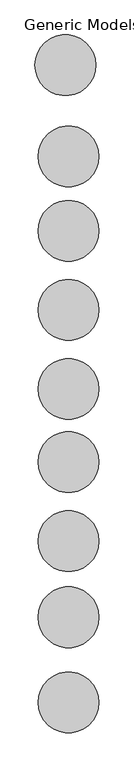
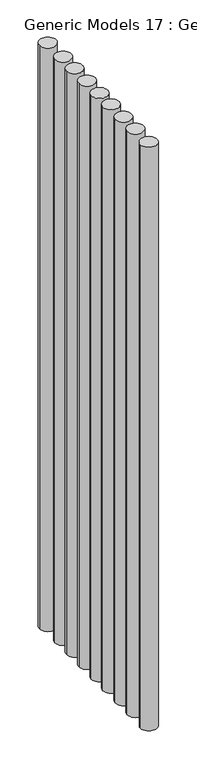
"""IFC4 building model written with IfcOpenShell, lengths in millimetres: proxy geometry, Generic Models 17 : Generic Models 17."""

from ifc_helpers import new_model, si_unit, point, frame, frame_2d, origin, place, context, project, spatial, circle_curve, trimmed, segment, composite_curve, outline, extrude, source, transform, mapped, element, save


def generic_models_17_generic_models_17_6d1cac68(model_context):
    return source(origin(), model_context, "Body", "SweptSolid", [
        extrude(outline(composite_curve([segment(trimmed(circle_curve(frame_2d((-2170.5790175, 11540.1337355)), 63.5), [point((-2234.0790175, 11540.1337355))], [point((-2107.0790175, 11540.1337355))], False, "CARTESIAN"), True, "CONTINUOUS"), segment(trimmed(circle_curve(frame_2d((-2170.5790175, 11540.1337355)), 63.5), [point((-2107.0790175, 11540.1337355))], [point((-2234.0790175, 11540.1337355))], False, "CARTESIAN"), True, "CONTINUOUS")], self_intersect=False)), frame((0.0, 0.0, 457.2), z_axis=(0.0, 0.0, 1.0), x_axis=(1.0, 0.0, 0.0)), (0.0, 0.0, 1.0), 4724.4),
        extrude(outline(composite_curve([segment(trimmed(circle_curve(frame_2d((-2163.9306633, 11349.749783)), 63.5), [point((-2227.4306633, 11349.749783))], [point((-2100.4306633, 11349.749783))], False, "CARTESIAN"), True, "CONTINUOUS"), segment(trimmed(circle_curve(frame_2d((-2163.9306633, 11349.749783)), 63.5), [point((-2100.4306633, 11349.749783))], [point((-2227.4306633, 11349.749783))], False, "CARTESIAN"), True, "CONTINUOUS")], self_intersect=False)), frame((0.0, 0.0, 457.2), z_axis=(0.0, 0.0, 1.0), x_axis=(1.0, 0.0, 0.0)), (0.0, 0.0, 1.0), 4724.4),
        extrude(outline(composite_curve([segment(trimmed(circle_curve(frame_2d((-2163.9306633, 11194.406573)), 63.5), [point((-2227.4306633, 11194.406573))], [point((-2100.4306633, 11194.406573))], False, "CARTESIAN"), True, "CONTINUOUS"), segment(trimmed(circle_curve(frame_2d((-2163.9306633, 11194.406573)), 63.5), [point((-2100.4306633, 11194.406573))], [point((-2227.4306633, 11194.406573))], False, "CARTESIAN"), True, "CONTINUOUS")], self_intersect=False)), frame((0.0, 0.0, 457.2), z_axis=(0.0, 0.0, 1.0), x_axis=(1.0, 0.0, 0.0)), (0.0, 0.0, 1.0), 4724.4),
        extrude(outline(composite_curve([segment(trimmed(circle_curve(frame_2d((-2163.9306633, 11029.306573)), 63.5), [point((-2227.4306633, 11029.306573))], [point((-2100.4306633, 11029.306573))], False, "CARTESIAN"), True, "CONTINUOUS"), segment(trimmed(circle_curve(frame_2d((-2163.9306633, 11029.306573)), 63.5), [point((-2100.4306633, 11029.306573))], [point((-2227.4306633, 11029.306573))], False, "CARTESIAN"), True, "CONTINUOUS")], self_intersect=False)), frame((0.0, 0.0, 457.2), z_axis=(0.0, 0.0, 1.0), x_axis=(1.0, 0.0, 0.0)), (0.0, 0.0, 1.0), 4724.4),
        extrude(outline(composite_curve([segment(trimmed(circle_curve(frame_2d((-2163.9306633, 10864.206573)), 63.5), [point((-2227.4306633, 10864.206573))], [point((-2100.4306633, 10864.206573))], False, "CARTESIAN"), True, "CONTINUOUS"), segment(trimmed(circle_curve(frame_2d((-2163.9306633, 10864.206573)), 63.5), [point((-2100.4306633, 10864.206573))], [point((-2227.4306633, 10864.206573))], False, "CARTESIAN"), True, "CONTINUOUS")], self_intersect=False)), frame((0.0, 0.0, 457.2), z_axis=(0.0, 0.0, 1.0), x_axis=(1.0, 0.0, 0.0)), (0.0, 0.0, 1.0), 4724.4),
        extrude(outline(composite_curve([segment(trimmed(circle_curve(frame_2d((-2163.9306633, 10711.806573)), 63.5), [point((-2227.4306633, 10711.806573))], [point((-2100.4306633, 10711.806573))], False, "CARTESIAN"), True, "CONTINUOUS"), segment(trimmed(circle_curve(frame_2d((-2163.9306633, 10711.806573)), 63.5), [point((-2100.4306633, 10711.806573))], [point((-2227.4306633, 10711.806573))], False, "CARTESIAN"), True, "CONTINUOUS")], self_intersect=False)), frame((0.0, 0.0, 457.2), z_axis=(0.0, 0.0, 1.0), x_axis=(1.0, 0.0, 0.0)), (0.0, 0.0, 1.0), 4724.4),
        extrude(outline(composite_curve([segment(trimmed(circle_curve(frame_2d((-2163.9306633, 10546.706573)), 63.5), [point((-2227.4306633, 10546.706573))], [point((-2100.4306633, 10546.706573))], False, "CARTESIAN"), True, "CONTINUOUS"), segment(trimmed(circle_curve(frame_2d((-2163.9306633, 10546.706573)), 63.5), [point((-2100.4306633, 10546.706573))], [point((-2227.4306633, 10546.706573))], False, "CARTESIAN"), True, "CONTINUOUS")], self_intersect=False)), frame((0.0, 0.0, 457.2), z_axis=(0.0, 0.0, 1.0), x_axis=(1.0, 0.0, 0.0)), (0.0, 0.0, 1.0), 4724.4),
        extrude(outline(composite_curve([segment(trimmed(circle_curve(frame_2d((-2163.9306633, 10387.956573)), 63.5), [point((-2227.4306633, 10387.956573))], [point((-2100.4306633, 10387.956573))], False, "CARTESIAN"), True, "CONTINUOUS"), segment(trimmed(circle_curve(frame_2d((-2163.9306633, 10387.956573)), 63.5), [point((-2100.4306633, 10387.956573))], [point((-2227.4306633, 10387.956573))], False, "CARTESIAN"), True, "CONTINUOUS")], self_intersect=False)), frame((0.0, 0.0, 457.2), z_axis=(0.0, 0.0, 1.0), x_axis=(1.0, 0.0, 0.0)), (0.0, 0.0, 1.0), 4724.4),
        extrude(outline(composite_curve([segment(trimmed(circle_curve(frame_2d((-2163.9306633, 10210.156573)), 63.5), [point((-2227.4306633, 10210.156573))], [point((-2100.4306633, 10210.156573))], False, "CARTESIAN"), True, "CONTINUOUS"), segment(trimmed(circle_curve(frame_2d((-2163.9306633, 10210.156573)), 63.5), [point((-2100.4306633, 10210.156573))], [point((-2227.4306633, 10210.156573))], False, "CARTESIAN"), True, "CONTINUOUS")], self_intersect=False)), frame((0.0, 0.0, 457.2), z_axis=(0.0, 0.0, 1.0), x_axis=(1.0, 0.0, 0.0)), (0.0, 0.0, 1.0), 4724.4),
    ])


if __name__ == "__main__":
    model = new_model("IFC4")
    model_context = context("Model", 3, world=origin())
    ifc_project = project(units=[si_unit("LENGTHUNIT", "METRE", prefix="MILLI")], contexts=[model_context])
    site = spatial("IfcSite", under=ifc_project)
    building = spatial("IfcBuilding", under=site)
    placement = place(None, origin())
    generic_models_17_generic_models_17_shape = generic_models_17_generic_models_17_6d1cac68(model_context)
    element("IfcBuildingElementProxy", 1, Name="Generic Models 17 : Generic Models 17", ObjectType="Generic Models 17 : Generic Models 17", at=placement, inside=building, context=model_context, shape_type="MappedRepresentation", body=[
        mapped(generic_models_17_generic_models_17_shape, transform((0.0, 0.0, 0.0), x_axis=(1.0, 0.0, 0.0), y_axis=(0.0, 1.0, 0.0), z_axis=(0.0, 0.0, 1.0))),
    ])
    save(model, "model.ifc")

# Revit data of these elements
# Element 1 (IfcBuildingElementProxy, "Generic Models 17 : Generic Models 17")
#   Materials on its faces: "Cherry"
# Materials
#   "Cherry": class "Wood", colour RGB 226 177 128, transparency 0, Description = "Prunus Serotina", Cost = 0
